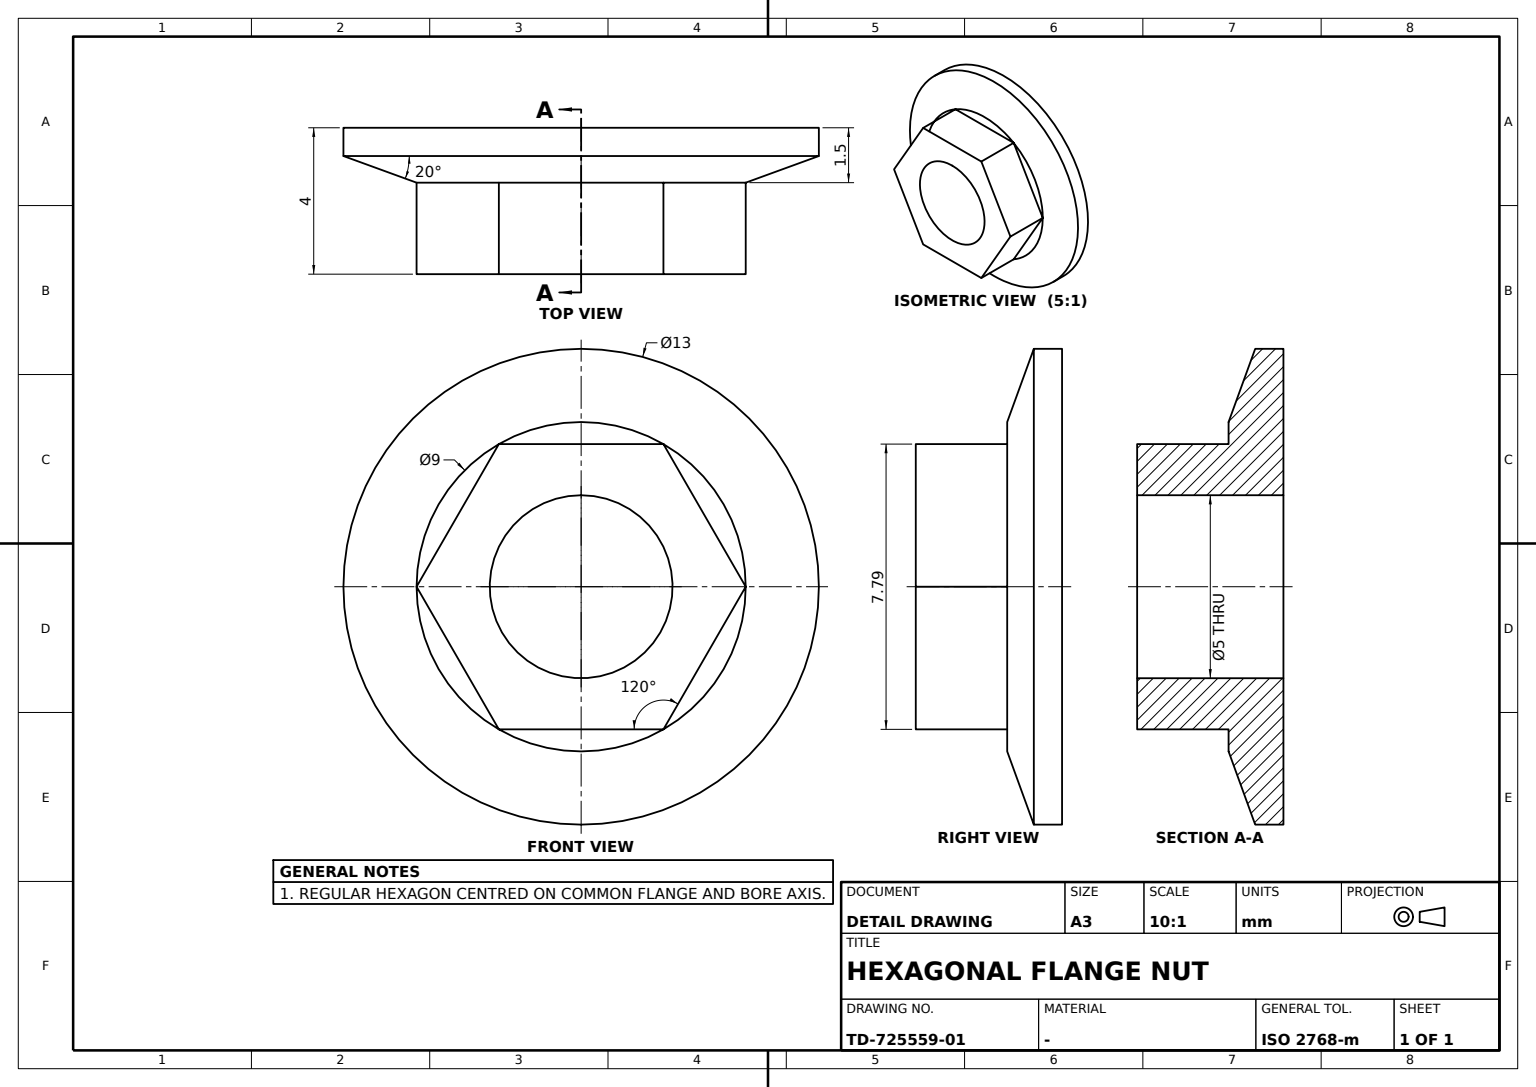
CATIA V5 part; units mm, degrees
sketch "Sketch1" plane through (0, 0, 0) normal (0, 0, 1) x (0, 1, 0)
  line L0 (0, 1.5) -> (0, 0)
  line L1 (0, 0) -> (6.5, 0)
  line L2 (6.5, 0) -> (6.5, 0.7721)
  line L3 (6.5, 0.7721) -> (4.5, 1.5)
  line L4 (4.5, 1.5) -> (0, 1.5)
  line L5 (6.5, 0.7721) -> (2.9677, 0.7721) construction
  dimension "angle L5 L3" = 20
  dimension "distance L4 L1" = 1.5
  dimension "length L4" = 4.5
  dimension "length L1" = 6.5
  constraint vertical L0 y-axis
  constraint vertical L2 y-axis
  constraint horizontal L1 x-axis
  constraint horizontal L4 x-axis
  constraint horizontal L5 x-axis
  constraint coincidence L0 y-axis
  constraint coincidence L1 x-axis
revolve "Shaft1" add sketch "Sketch1" angle 360 about axis through (0, 0, 0) along (1, 0, 0)
sketch "Sketch2" plane through (-1.5, 0, 0) normal (-1, 0, 0) x (0, -1, 0)
  point P0 (-2.25, -3.8971)
  point P1 (2.25, -3.8971)
  point P2 (4.5, 0)
  point P3 (2.25, 3.8971)
  point P4 (-2.25, 3.8971)
  point P5 (-4.5, 0)
  point P6 (0, -3.8971)
  line L0 (-2.25, -3.8971) -> (2.25, -3.8971)
  line L1 (2.25, -3.8971) -> (4.5, 0)
  line L2 (4.5, 0) -> (2.25, 3.8971)
  line L3 (2.25, 3.8971) -> (-2.25, 3.8971)
  line L4 (-2.25, 3.8971) -> (-4.5, 0)
  line L5 (-4.5, 0) -> (-2.25, -3.8971)
  line L6 (0, 0) -> (0, -3.8971) construction
  circle A0 centre (0, 0) radius 4.5 construction
  arc A1 (2.25, 3.8971) -> (-4.5, 0) centre (-2.25, 3.8971) cw construction
  arc A2 (4.5, 0) -> (-2.25, -3.8971) centre (2.25, -3.8971) ccw construction
  dimension "distance P5 P2" = 9
  constraint vertical L6 y-axis
  constraint coincidence A0 P0
  constraint coincidence A0 P1
  constraint coincidence A0 P2
  constraint coincidence A0 P3
  constraint coincidence A0 P4
  constraint coincidence A0 P5
  constraint coincidence A1 origin
  constraint coincidence A2 origin
  constraint midpoint P6 L0
  constraint parallelism L0 L3
extrude "Pad1" add sketch "Sketch2" along normal blind 2.5
sketch "Sketch3" plane through (-4, 0, 0) normal (-1, 0, 0) x (0, -1, 0)
  circle A0 centre (0, 0) radius 2.5
  point P0 (0, 0)
  dimension "radius A0" = 2.5
  constraint coincidence P0 y-axis
  constraint coincidence P0 origin
extrude "Pocket1" cut sketch "Sketch3" against normal through all
